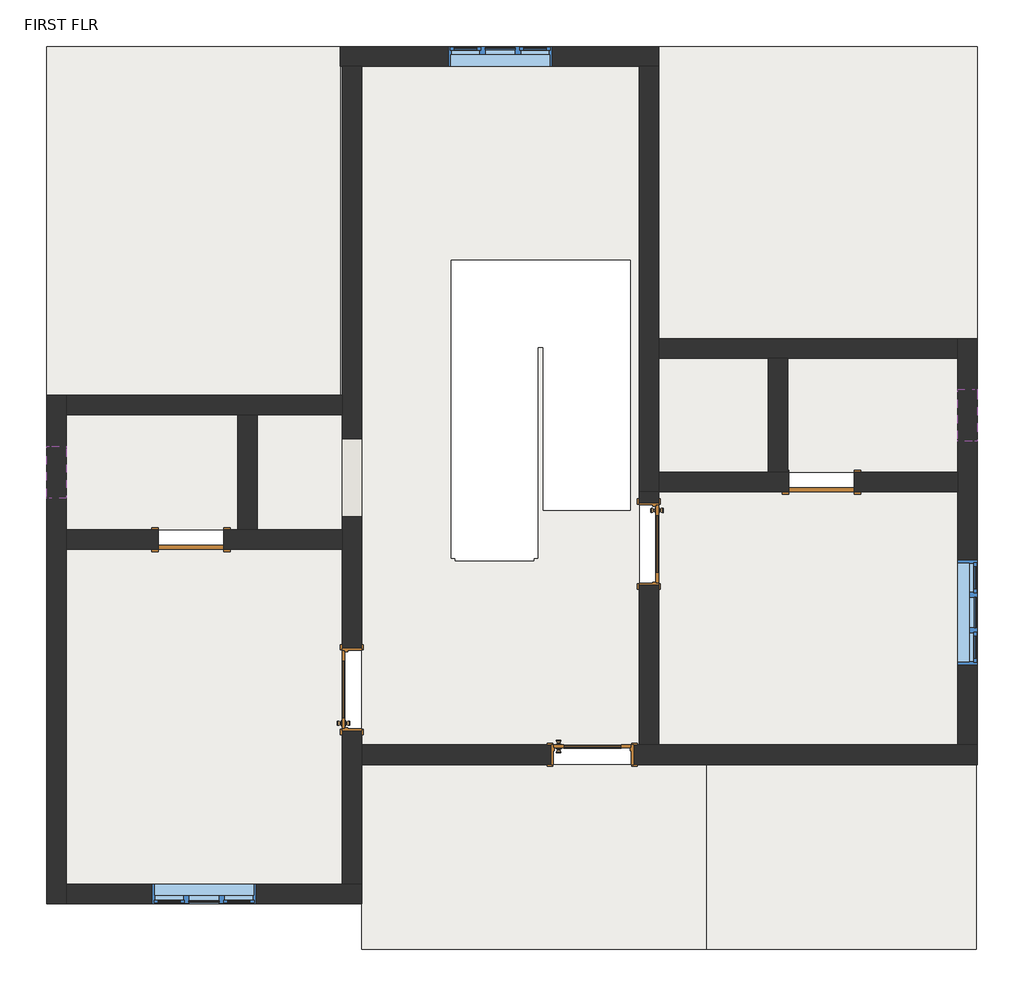
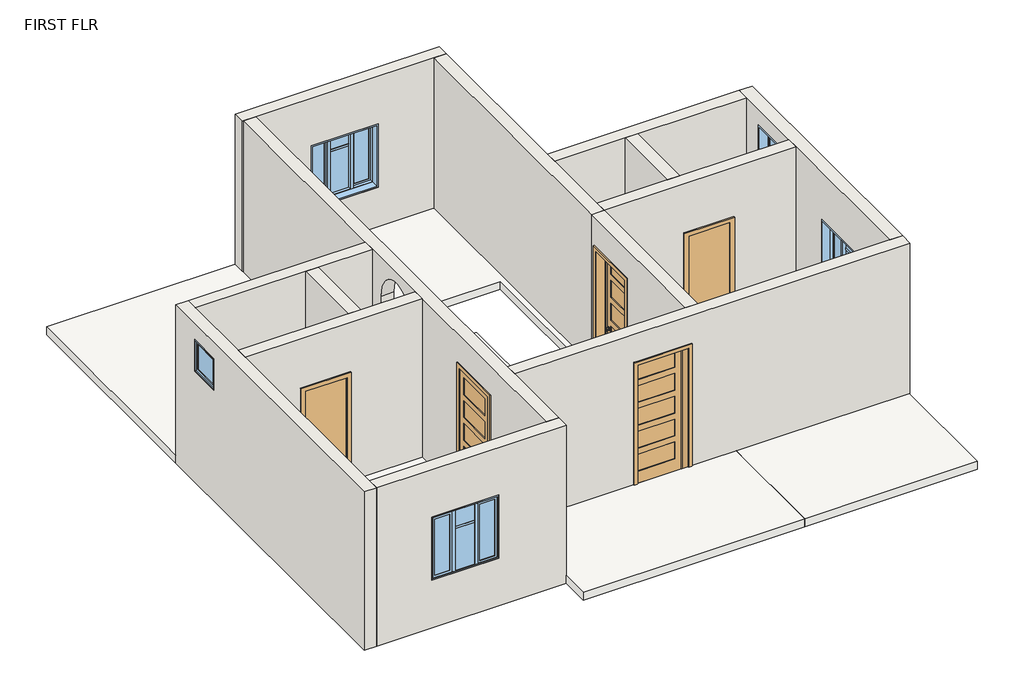
# One storey, incomplete: 14 walls, 8 slabs, 5 doors, 5 windows.
"""IFC4 building model written with IfcOpenShell, lengths in millimetres."""

from ifc_helpers import new_model, si_unit, point, frame, origin, place, context, project, spatial, polyline, ellipse_curve, trimmed, outline, extrude, faceted_brep, transform, mapped, element, save
from ifc_brep_helpers import plane_surface, extruded_surface, advanced_brep
from components import door_d793c26e, door_a1484949, window_80340324, window_casement_triple_middle_transom_window_4_x_4_1416bf83

model = new_model("IFC4")

# Units and contexts
model_context = context("Model", 3, world=origin())
ifc_project = project(units=[si_unit("LENGTHUNIT", "METRE", prefix="MILLI")], contexts=[model_context])

# Site, building, storey
site = spatial("IfcSite", under=ifc_project)
building = spatial("IfcBuilding", under=site)
storey = spatial("IfcBuildingStorey", under=building, Name="FIRST FLR", Elevation=3657.6)

# Doors
placement = place(None, origin())
door_shape = door_d793c26e(model_context)
element("IfcDoor", 1, ObjectType="Door-Interior-Single-5_Panel_Vert-Wood : 36\" x 96\"", at=placement, inside=storey, context=model_context, shape_type="MappedRepresentation", body=[
    mapped(door_shape, transform((-5771.8431792, -6106.9198807, 3657.6), x_axis=(1.0, 0.0, 0.0), y_axis=(0.0, 1.0, 0.0), z_axis=(0.0, 0.0, 1.0))),
])
element("IfcDoor", 2, ObjectType="Door-Interior-Single-5_Panel_Vert-Wood : 36\" x 96\"", at=placement, inside=storey, context=model_context, shape_type="MappedRepresentation", body=[
    mapped(door_shape, transform((-8587.0956632, -5348.0948807, 3657.6), x_axis=(0.0, 1.0, 0.0), y_axis=(-1.0, 0.0, 0.0), z_axis=(0.0, 0.0, 1.0))),
])
element("IfcDoor", 3, ObjectType="Door-Interior-Single-5_Panel_Vert-Wood : 36\" x 96\"", at=placement, inside=storey, context=model_context, shape_type="MappedRepresentation", body=[
    mapped(door_shape, transform((-5108.2681792, -3646.2948807, 3657.6), x_axis=(0.0, -1.0, 0.0), y_axis=(1.0, 0.0, 0.0), z_axis=(0.0, 0.0, 1.0))),
])
door_2_shape = door_a1484949(model_context)
element("IfcDoor", 4, ObjectType="Single-Flush : 30\" x 80\"", at=placement, inside=storey, context=model_context, shape_type="MappedRepresentation", body=[
    mapped(door_2_shape, transform((-10463.5206632, -3595.4948807, 3657.6), x_axis=(-1.0, 0.0, 0.0), y_axis=(0.0, -1.0, 0.0), z_axis=(0.0, 0.0, 1.0))),
])
element("IfcDoor", 5, ObjectType="Single-Flush : 30\" x 80\"", at=placement, inside=storey, context=model_context, shape_type="MappedRepresentation", body=[
    mapped(door_2_shape, transform((-3092.1431792, -2922.3948807, 3657.6), x_axis=(-1.0, 0.0, 0.0), y_axis=(0.0, -1.0, 0.0), z_axis=(0.0, 0.0, 1.0))),
])

# Slabs
element("IfcSlab", 6, ObjectType="GENERIC 6\"", at=placement, inside=storey, context=model_context, shape_type="SweptSolid", body=[
    extrude(outline(polyline([(-8698.2206632, -3709.7948807), (-8698.2206632, -7621.3948807), (-11924.0206632, -7621.3948807), (-11924.0206632, -3709.7948807), (-8698.2206632, -3709.7948807)])), frame((0.0, 0.0, 3505.2), z_axis=(0.0, 0.0, 1.0), x_axis=(1.0, 0.0, 0.0)), (0.0, 0.0, 1.0), 152.4),
])
element("IfcSlab", 7, ObjectType="GENERIC 6\"", at=placement, inside=storey, context=model_context, shape_type="SweptSolid", body=[
    extrude(outline(polyline([(-9917.4206632, -2134.9948807), (-9917.4206632, -3481.1948807), (-11924.0206632, -3481.1948807), (-11924.0206632, -2134.9948807), (-9917.4206632, -2134.9948807)])), frame((0.0, 0.0, 3505.2), z_axis=(0.0, 0.0, 1.0), x_axis=(1.0, 0.0, 0.0)), (0.0, 0.0, 1.0), 152.4),
])
element("IfcSlab", 8, ObjectType="GENERIC 6\"", at=placement, inside=storey, context=model_context, shape_type="SweptSolid", body=[
    extrude(outline(polyline([(-8698.2206632, -2134.9948807), (-8698.2206632, -3481.1948807), (-9688.8206632, -3481.1948807), (-9688.8206632, -2134.9948807), (-8698.2206632, -2134.9948807)])), frame((0.0, 0.0, 3505.2), z_axis=(0.0, 0.0, 1.0), x_axis=(1.0, 0.0, 0.0)), (0.0, 0.0, 1.0), 152.4),
])
element("IfcSlab", 9, ObjectType="GENERIC 6\"", at=placement, inside=storey, context=model_context, shape_type="SweptSolid", body=[
    extrude(outline(polyline([(-5225.7431792, 1941.7051193), (-5225.7431792, -5995.7948807), (-8469.6206632, -5995.7948807), (-8469.6206632, 1941.7051193), (-5225.7431792, 1941.7051193)]), holes=[polyline([(-5329.6481169, -329.5249317), (-7422.8431792, -329.5249317), (-7422.8431792, -3809.3249317), (-7372.0431792, -3809.3249317), (-7372.0431792, -3841.0749317), (-6457.6431792, -3841.0749317), (-6457.6431792, -3809.3249317), (-6406.8431792, -3809.3249317), (-6406.8431792, -1345.5249317), (-6345.6481169, -1345.5249317), (-6345.6481169, -3250.5249317), (-5329.6481169, -3250.5249317), (-5329.6481169, -329.5249317)])]), frame((0.0, 0.0, 3657.6), z_axis=(0.0, 0.0, 1.0), x_axis=(1.0, 0.0, 0.0)), (0.0, 0.0, 1.0), 152.4),
    extrude(outline(polyline([(-1497.3206632, -3036.6948807), (-1497.3206632, -5995.7948807), (-4997.1431792, -5995.7948807), (-4997.1431792, -3036.6948807), (-1497.3206632, -3036.6948807)])), frame((0.0, 0.0, 3657.6), z_axis=(0.0, 0.0, 1.0), x_axis=(1.0, 0.0, 0.0)), (0.0, 0.0, 1.0), 152.4),
    extrude(outline(polyline([(-4431.0206632, -6224.3948807), (-4431.0206632, -8383.3948807), (-8469.6206632, -8383.3948807), (-8469.6206632, -6224.3948807), (-4431.0206632, -6224.3948807)])), frame((0.0, 0.0, 3657.6), z_axis=(0.0, 0.0, 1.0), x_axis=(1.0, 0.0, 0.0)), (0.0, 0.0, 1.0), 152.4),
])
element("IfcSlab", 10, ObjectType="GENERIC 6\"", at=placement, inside=storey, context=model_context, shape_type="SweptSolid", body=[
    extrude(outline(polyline([(-1497.3206632, -1474.5948807), (-1497.3206632, -2808.0948807), (-3485.8431792, -2808.0948807), (-3485.8431792, -1474.5948807), (-1497.3206632, -1474.5948807)])), frame((0.0, 0.0, 3505.2), z_axis=(0.0, 0.0, 1.0), x_axis=(1.0, 0.0, 0.0)), (0.0, 0.0, 1.0), 152.4),
    extrude(outline(polyline([(-3714.4431792, -1474.5948807), (-3714.4431792, -2808.0948807), (-4997.1431792, -2808.0948807), (-4997.1431792, -1474.5948807), (-3714.4431792, -1474.5948807)])), frame((0.0, 0.0, 3505.2), z_axis=(0.0, 0.0, 1.0), x_axis=(1.0, 0.0, 0.0)), (0.0, 0.0, 1.0), 152.4),
])
element("IfcSlab", 11, ObjectType="GENERIC 6\"", at=placement, inside=storey, context=model_context, shape_type="SweptSolid", body=[
    extrude(outline(polyline([(-12152.6206632, 2170.3051193), (-8718.2431792, 2170.3051193), (-8718.2431792, -1906.3948807), (-12152.6206632, -1906.3948807), (-12152.6206632, 2170.3051193)])), frame((0.0, 0.0, 3657.6), z_axis=(0.0, 0.0, 1.0), x_axis=(1.0, 0.0, 0.0)), (0.0, 0.0, 1.0), 152.4),
])
element("IfcSlab", 12, ObjectType="GENERIC 6\"", at=placement, inside=storey, context=model_context, shape_type="SweptSolid", body=[
    extrude(outline(polyline([(-1268.7206632, 2170.3051193), (-1268.7206632, -1245.9948807), (-4997.1431792, -1245.9948807), (-4997.1431792, 2170.3051193), (-1268.7206632, 2170.3051193)])), frame((0.0, 0.0, 3657.6), z_axis=(0.0, 0.0, 1.0), x_axis=(1.0, 0.0, 0.0)), (0.0, 0.0, 1.0), 152.4),
])
element("IfcSlab", 13, ObjectType="GENERIC 6\"", at=placement, inside=storey, context=model_context, shape_type="SweptSolid", body=[
    extrude(outline(polyline([(-1281.4206632, -6224.3948807), (-1281.4206632, -8383.3948807), (-4431.0206632, -8383.3948807), (-4431.0206632, -6224.3948807), (-1281.4206632, -6224.3948807)])), frame((0.0, 0.0, 3657.6), z_axis=(0.0, 0.0, 1.0), x_axis=(1.0, 0.0, 0.0)), (0.0, 0.0, 1.0), 152.4),
])

# Walls
element("IfcWall", 14, ObjectType="WALL 9\"", at=placement, inside=storey, context=model_context, shape_type="Brep", body=[
    faceted_brep([(-11924.0206632, -7849.9948807, 3657.6), (-11924.0206632, -7621.3948807, 3657.6), (-11924.0206632, -3709.7948807, 3657.6), (-11924.0206632, -3481.1948807, 3657.6), (-11924.0206632, -2134.9948807, 3657.6), (-11924.0206632, -1906.3948807, 3657.6), (-11924.0206632, -1906.3948807, 6705.6), (-11924.0206632, -2134.9948807, 6705.6), (-11924.0206632, -3481.1948807, 6705.6), (-11924.0206632, -3709.7948807, 6705.6), (-11924.0206632, -7621.3948807, 6705.6), (-11924.0206632, -7849.9948807, 6705.6), (-11924.0206632, -2503.2948807, 6400.8), (-11924.0206632, -2503.2948807, 5791.2), (-11924.0206632, -3112.8948807, 5791.2), (-11924.0206632, -3112.8948807, 6400.8), (-12152.6206632, -7849.9948807, 3657.6), (-12152.6206632, -7849.9948807, 6705.6), (-12152.6206632, -1906.3948807, 6705.6), (-12152.6206632, -1906.3948807, 3657.6), (-12152.6206632, -2503.2948807, 6400.8), (-12152.6206632, -3112.8948807, 6400.8), (-12152.6206632, -3112.8948807, 5791.2), (-12152.6206632, -2503.2948807, 5791.2)], [[[0, 1, 2, 3, 4, 5, 6, 7, 8, 9, 10, 11], [12, 13, 14, 15]], [[16, 17, 18, 19], [20, 21, 22, 23]], [[5, 4, 3, 2, 1, 0, 16, 19]], [[11, 10, 9, 8, 7, 6, 18, 17]], [[0, 11, 17, 16]], [[6, 5, 19, 18]], [[13, 12, 20, 23]], [[14, 13, 23, 22]], [[15, 14, 22, 21]], [[12, 15, 21, 20]]]),
])
element("IfcWall", 15, ObjectType="WALL 9\"", at=placement, inside=storey, context=model_context, shape_type="Brep", body=[
    faceted_brep([(-11924.0206632, -7849.9948807, 3657.6), (-8469.6206632, -7849.9948807, 3657.6), (-8469.6206632, -7849.9948807, 6705.6), (-11924.0206632, -7849.9948807, 6705.6), (-10920.7206632, -7849.9948807, 5791.2), (-9701.5206632, -7849.9948807, 5791.2), (-9701.5206632, -7849.9948807, 4572.0), (-10920.7206632, -7849.9948807, 4572.0), (-11924.0206632, -7621.3948807, 3657.6), (-11924.0206632, -7621.3948807, 6705.6), (-8698.2206632, -7621.3948807, 6705.6), (-8469.6206632, -7621.3948807, 6705.6), (-8469.6206632, -7621.3948807, 3657.6), (-8698.2206632, -7621.3948807, 3657.6), (-10920.7206632, -7621.3948807, 5791.2), (-10920.7206632, -7621.3948807, 4572.0), (-9701.5206632, -7621.3948807, 4572.0), (-9701.5206632, -7621.3948807, 5791.2)], [[[0, 1, 2, 3], [4, 5, 6, 7]], [[8, 9, 10, 11, 12, 13], [14, 15, 16, 17]], [[1, 0, 8, 13, 12]], [[3, 2, 11, 10, 9]], [[0, 3, 9, 8]], [[2, 1, 12, 11]], [[15, 14, 4, 7]], [[16, 15, 7, 6]], [[17, 16, 6, 5]], [[14, 17, 5, 4]]]),
])
element("IfcWall", 16, ObjectType="WALL 9\"", at=placement, inside=storey, context=model_context, shape_type="Brep", body=[
    faceted_brep([(-11924.0206632, -2134.9948807, 3657.6), (-9917.4206632, -2134.9948807, 3657.6), (-9688.8206632, -2134.9948807, 3657.6), (-8698.2206632, -2134.9948807, 3657.6), (-8698.2206632, -2134.9948807, 6705.6), (-9688.8206632, -2134.9948807, 6705.6), (-9917.4206632, -2134.9948807, 6705.6), (-11924.0206632, -2134.9948807, 6705.6), (-11924.0206632, -1906.3948807, 3657.6), (-11924.0206632, -1906.3948807, 6705.6), (-8698.2206632, -1906.3948807, 6705.6), (-8698.2206632, -1906.3948807, 3657.6)], [[[0, 1, 2, 3, 4, 5, 6, 7]], [[8, 9, 10, 11]], [[3, 2, 1, 0, 8, 11]], [[7, 6, 5, 4, 10, 9]], [[0, 7, 9, 8]], [[4, 3, 11, 10]]]),
])
element("IfcWall", 17, ObjectType="WALL 9\"", at=placement, inside=storey, context=model_context, shape_type="Brep", body=[
    faceted_brep([(-11924.0206632, -3709.7948807, 3657.6), (-10844.5206632, -3709.7948807, 3657.6), (-10844.5206632, -3709.7948807, 5689.6), (-10082.5206632, -3709.7948807, 5689.6), (-10082.5206632, -3709.7948807, 3657.6), (-8698.2206632, -3709.7948807, 3657.6), (-8698.2206632, -3709.7948807, 6705.6), (-11924.0206632, -3709.7948807, 6705.6), (-10844.5206632, -3481.1948807, 5689.6), (-10844.5206632, -3481.1948807, 3657.6), (-11924.0206632, -3481.1948807, 3657.6), (-11924.0206632, -3481.1948807, 6705.6), (-9917.4206632, -3481.1948807, 6705.6), (-9688.8206632, -3481.1948807, 6705.6), (-8698.2206632, -3481.1948807, 6705.6), (-8698.2206632, -3481.1948807, 3657.6), (-9688.8206632, -3481.1948807, 3657.6), (-9917.4206632, -3481.1948807, 3657.6), (-10082.5206632, -3481.1948807, 3657.6), (-10082.5206632, -3481.1948807, 5689.6)], [[[0, 1, 2, 3, 4, 5, 6, 7]], [[8, 9, 10, 11, 12, 13, 14, 15, 16, 17, 18, 19]], [[10, 9, 1, 0]], [[18, 17, 16, 15, 5, 4]], [[7, 6, 14, 13, 12, 11]], [[0, 7, 11, 10]], [[6, 5, 15, 14]], [[2, 1, 9, 8]], [[3, 2, 8, 19]], [[4, 3, 19, 18]]]),
])
element("IfcWall", 18, ObjectType="WALL 9\"", at=placement, inside=storey, context=model_context, shape_type="SweptSolid", body=[
    extrude(outline(polyline([(-9917.4206632, -3481.1948807), (-9917.4206632, -2134.9948807), (-9688.8206632, -2134.9948807), (-9688.8206632, -3481.1948807), (-9917.4206632, -3481.1948807)])), frame((0.0, 0.0, 3657.6), z_axis=(0.0, 0.0, 1.0), x_axis=(1.0, 0.0, 0.0)), (0.0, 0.0, 1.0), 3048.0),
])
element("IfcWall", 19, ObjectType="WALL 9\"", at=placement, inside=storey, context=model_context, shape_type="AdvancedBrep", body=[
    advanced_brep(
    [(-8469.6206632, 1941.7051193, 6705.6), (-8469.6206632, -5995.7948807, 6705.6), (-8469.6206632, -6224.3948807, 6705.6), (-8469.6206632, -7621.3948807, 6705.6), (-8469.6206632, -7621.3948807, 3657.6), (-8469.6206632, -6224.3948807, 3657.6), (-8469.6206632, -5995.7948807, 3657.6), (-8469.6206632, -5830.6948807, 3657.6), (-8469.6206632, -5830.6948807, 6121.4), (-8469.6206632, -4865.4948807, 6121.4), (-8469.6206632, -4865.4948807, 3657.6), (-8469.6206632, 1941.7051193, 3657.6), (-8469.6206632, -3327.8747617, 5972.3014733), (-8469.6206632, -2413.4747617, 5972.3014733), (-8469.6206632, -2413.4747617, 3838.7014733), (-8469.6206632, -3327.8747617, 3838.7014733), (-8698.2206632, -7621.3948807, 6705.6), (-8698.2206632, -3709.7948807, 6705.6), (-8698.2206632, -3481.1948807, 6705.6), (-8698.2206632, -2134.9948807, 6705.6), (-8698.2206632, -1906.3948807, 6705.6), (-8698.2206632, 1941.7051193, 6705.6), (-8698.2206632, 1941.7051193, 3657.6), (-8698.2206632, -1906.3948807, 3657.6), (-8698.2206632, -2134.9948807, 3657.6), (-8698.2206632, -3481.1948807, 3657.6), (-8698.2206632, -3709.7948807, 3657.6), (-8698.2206632, -4865.4948807, 3657.6), (-8698.2206632, -4865.4948807, 6121.4), (-8698.2206632, -5830.6948807, 6121.4), (-8698.2206632, -5830.6948807, 3657.6), (-8698.2206632, -7621.3948807, 3657.6), (-8698.2206632, -2413.4747617, 5972.3014733), (-8698.2206632, -3327.8747617, 5972.3014733), (-8698.2206632, -3327.8747617, 3838.7014733), (-8698.2206632, -2413.4747617, 3838.7014733)],
    [
        (0, 1),
        (1, 2),
        (2, 3),
        (3, 4),
        (4, 5),
        (5, 6),
        (6, 7),
        (7, 8),
        (8, 9),
        (9, 10),
        (10, 11),
        (11, 0),
        (12, 13, ellipse_curve(frame((-8469.6206632, -2870.6747617, 5972.3014733), z_axis=(-1.0, 0.0, 0.0), x_axis=(0.0, 0.0, -1.0)), 533.4, 457.2)),
        (13, 14),
        (14, 15),
        (15, 12),
        (16, 17),
        (17, 18),
        (18, 19),
        (19, 20),
        (20, 21),
        (21, 22),
        (22, 23),
        (23, 24),
        (24, 25),
        (25, 26),
        (26, 27),
        (27, 28),
        (28, 29),
        (29, 30),
        (30, 31),
        (31, 16),
        (32, 33, ellipse_curve(frame((-8698.2206632, -2870.6747617, 5972.3014733), z_axis=(1.0, 0.0, 0.0), x_axis=(0.0, 0.0, -1.0)), 533.4, 457.2)),
        (33, 34),
        (34, 35),
        (35, 32),
        (3, 16),
        (31, 4),
        (11, 22),
        (21, 0),
        (9, 28),
        (27, 10),
        (8, 29),
        (7, 30),
        (12, 33),
        (32, 13),
        (35, 14),
        (34, 15),
    ],
    [
        plane_surface(frame((-8469.6206632, -7621.3948807, 3657.6), z_axis=(1.0, 0.0, 0.0), x_axis=(0.0, 1.0, 0.0))),
        plane_surface(frame((-8698.2206632, -7621.3948807, 3657.6), z_axis=(-1.0, 0.0, 0.0), x_axis=(0.0, -1.0, 0.0))),
        plane_surface(frame((-11924.0206632, -7621.3948807, 3657.6), z_axis=(0.0, -1.0, 0.0), x_axis=(-1.0, 0.0, 0.0))),
        plane_surface(frame((-8703.812186, 1941.7051193, 3657.6), z_axis=(0.0, 1.0, 0.0), x_axis=(1.0, 0.0, 0.0))),
        plane_surface(frame((-6945.6206632, -4865.4948807, 3657.6), z_axis=(0.0, -1.0, 0.0), x_axis=(-1.0, 0.0, 0.0))),
        plane_surface(frame((-6945.6206632, -4865.4948807, 6121.4), z_axis=(0.0, 0.0, -1.0), x_axis=(-1.0, 0.0, 0.0))),
        plane_surface(frame((-6945.6206632, -5830.6948807, 6121.4), z_axis=(0.0, 1.0, 0.0), x_axis=(-1.0, 0.0, 0.0))),
        plane_surface(frame((-8469.6206632, -7735.6948807, 3657.6), z_axis=(0.0, 0.0, -1.0), x_axis=(-1.0, 0.0, 0.0))),
        plane_surface(frame((-8469.6206632, 2056.0051193, 6705.6), z_axis=(0.0, 0.0, 1.0), x_axis=(-1.0, 0.0, 0.0))),
        extruded_surface(trimmed(ellipse_curve(frame((-8812.5206632, -2870.6747617, 5972.3014733), z_axis=(-1.0, 0.0, 0.0), x_axis=(0.0, 1.0, 0.0)), 457.2, 533.4), [point((-8812.5206632, -3327.8747617, 5972.3014733))], [point((-8812.5206632, -2413.4747617, 5972.3014733))], True, "CARTESIAN"), (228.60000000000036, 0.0, 0.0), 228.60000000000036),
        plane_surface(frame((-8469.6206632, -2413.4747617, 5972.3014733), z_axis=(0.0, -1.0, 0.0), x_axis=(-1.0, 0.0, 0.0))),
        plane_surface(frame((-8469.6206632, -2413.4747617, 3838.7014733), z_axis=(0.0, 0.0, 1.0), x_axis=(-1.0, 0.0, 0.0))),
        plane_surface(frame((-8469.6206632, -3327.8747617, 3838.7014733), z_axis=(0.0, 1.0, 0.0), x_axis=(-1.0, 0.0, 0.0))),
    ],
    [
        (0, [[1, 2, 3, 4, 5, 6, 7, 8, 9, 10, 11, 12], [13, 14, 15, 16]]),
        (1, [[17, 18, 19, 20, 21, 22, 23, 24, 25, 26, 27, 28, 29, 30, 31, 32], [33, 34, 35, 36]]),
        (2, [[-4, 37, -32, 38]]),
        (3, [[-12, 39, -22, 40]]),
        (4, [[41, -28, 42, -10]]),
        (5, [[-41, -9, 43, -29]]),
        (6, [[-43, -8, 44, -30]]),
        (7, [[-38, -31, -44, -7, -6, -5]]),
        (7, [[-39, -11, -42, -27, -26, -25, -24, -23]]),
        (8, [[-3, -2, -1, -40, -21, -20, -19, -18, -17, -37]]),
        (9, [[-13, 45, -33, 46]]),
        (10, [[-14, -46, -36, 47]]),
        (11, [[-15, -47, -35, 48]]),
        (12, [[-16, -48, -34, -45]]),
    ],
),
])
element("IfcWall", 20, ObjectType="WALL 9\"", at=placement, inside=storey, context=model_context, shape_type="Brep", body=[
    faceted_brep([(-8718.2431792, 1941.7051193, 3657.6), (-8698.2206632, 1941.7051193, 3657.6), (-8469.6206632, 1941.7051193, 3657.6), (-5225.7431792, 1941.7051193, 3657.6), (-4997.1431792, 1941.7051193, 3657.6), (-4997.1431792, 1941.7051193, 6705.6), (-5225.7431792, 1941.7051193, 6705.6), (-8469.6206632, 1941.7051193, 6705.6), (-8698.2206632, 1941.7051193, 6705.6), (-8718.2431792, 1941.7051193, 6705.6), (-6238.0819212, 1941.7051193, 5791.2), (-6238.0819212, 1941.7051193, 4572.0), (-7457.2819212, 1941.7051193, 4572.0), (-7457.2819212, 1941.7051193, 5791.2), (-8718.2431792, 2170.3051193, 3657.6), (-8718.2431792, 2170.3051193, 6705.6), (-4997.1431792, 2170.3051193, 6705.6), (-4997.1431792, 2170.3051193, 3657.6), (-6238.0819212, 2170.3051193, 5791.2), (-7457.2819212, 2170.3051193, 5791.2), (-7457.2819212, 2170.3051193, 4572.0), (-6238.0819212, 2170.3051193, 4572.0)], [[[0, 1, 2, 3, 4, 5, 6, 7, 8, 9], [10, 11, 12, 13]], [[14, 15, 16, 17], [18, 19, 20, 21]], [[4, 3, 2, 1, 0, 14, 17]], [[9, 8, 7, 6, 5, 16, 15]], [[0, 9, 15, 14]], [[5, 4, 17, 16]], [[11, 10, 18, 21]], [[12, 11, 21, 20]], [[13, 12, 20, 19]], [[10, 13, 19, 18]]]),
])
element("IfcWall", 21, ObjectType="WALL 9\"", at=placement, inside=storey, context=model_context, shape_type="Brep", body=[
    faceted_brep([(-5225.7431792, 1941.7051193, 3657.6), (-5225.7431792, -3036.6948807, 3657.6), (-5225.7431792, -3036.6948807, 6705.6), (-5225.7431792, 1941.7051193, 6705.6), (-4997.1431792, 1941.7051193, 3657.6), (-4997.1431792, 1941.7051193, 6705.6), (-4997.1431792, -1245.9948807, 6705.6), (-4997.1431792, -1474.5948807, 6705.6), (-4997.1431792, -2808.0948807, 6705.6), (-4997.1431792, -3036.6948807, 6705.6), (-4997.1431792, -3036.6948807, 3657.6), (-4997.1431792, -2808.0948807, 3657.6), (-4997.1431792, -1474.5948807, 3657.6), (-4997.1431792, -1245.9948807, 3657.6)], [[[0, 1, 2, 3]], [[4, 5, 6, 7, 8, 9, 10, 11, 12, 13]], [[1, 0, 4, 13, 12, 11, 10]], [[3, 2, 9, 8, 7, 6, 5]], [[0, 3, 5, 4]], [[2, 1, 10, 9]]]),
])
element("IfcWall", 22, ObjectType="WALL 9\"", at=placement, inside=storey, context=model_context, shape_type="Brep", body=[
    faceted_brep([(-1268.7206632, -6224.3948807, 6705.6), (-8469.6206632, -6224.3948807, 6705.6), (-8469.6206632, -6224.3948807, 3657.6), (-6254.4431792, -6224.3948807, 3657.6), (-6254.4431792, -6224.3948807, 6121.4), (-5289.2431792, -6224.3948807, 6121.4), (-5289.2431792, -6224.3948807, 3657.6), (-1268.7206632, -6224.3948807, 3657.6), (-8469.6206632, -5995.7948807, 6705.6), (-5225.7431792, -5995.7948807, 6705.6), (-4997.1431792, -5995.7948807, 6705.6), (-1497.3206632, -5995.7948807, 6705.6), (-1268.7206632, -5995.7948807, 6705.6), (-1268.7206632, -5995.7948807, 3657.6), (-1497.3206632, -5995.7948807, 3657.6), (-4997.1431792, -5995.7948807, 3657.6), (-5225.7431792, -5995.7948807, 3657.6), (-5289.2431792, -5995.7948807, 3657.6), (-5289.2431792, -5995.7948807, 6121.4), (-6254.4431792, -5995.7948807, 6121.4), (-6254.4431792, -5995.7948807, 3657.6), (-8469.6206632, -5995.7948807, 3657.6)], [[[0, 1, 2, 3, 4, 5, 6, 7]], [[8, 9, 10, 11, 12, 13, 14, 15, 16, 17, 18, 19, 20, 21]], [[2, 21, 20, 3]], [[13, 7, 6, 17, 16, 15, 14]], [[1, 0, 12, 11, 10, 9, 8]], [[2, 1, 8, 21]], [[0, 7, 13, 12]], [[5, 18, 17, 6]], [[18, 5, 4, 19]], [[19, 4, 3, 20]]]),
])
element("IfcWall", 23, ObjectType="WALL 9\"", at=placement, inside=storey, context=model_context, shape_type="Brep", body=[
    faceted_brep([(-4997.1431792, -3036.6948807, 3657.6), (-3473.1431792, -3036.6948807, 3657.6), (-3473.1431792, -3036.6948807, 5689.6), (-2711.1431792, -3036.6948807, 5689.6), (-2711.1431792, -3036.6948807, 3657.6), (-1497.3206632, -3036.6948807, 3657.6), (-1497.3206632, -3036.6948807, 6705.6), (-4997.1431792, -3036.6948807, 6705.6), (-3473.1431792, -2808.0948807, 5689.6), (-3473.1431792, -2808.0948807, 3657.6), (-3485.8431792, -2808.0948807, 3657.6), (-3714.4431792, -2808.0948807, 3657.6), (-4997.1431792, -2808.0948807, 3657.6), (-4997.1431792, -2808.0948807, 6705.6), (-3714.4431792, -2808.0948807, 6705.6), (-3485.8431792, -2808.0948807, 6705.6), (-1497.3206632, -2808.0948807, 6705.6), (-1497.3206632, -2808.0948807, 3657.6), (-2711.1431792, -2808.0948807, 3657.6), (-2711.1431792, -2808.0948807, 5689.6)], [[[0, 1, 2, 3, 4, 5, 6, 7]], [[8, 9, 10, 11, 12, 13, 14, 15, 16, 17, 18, 19]], [[18, 17, 5, 4]], [[12, 11, 10, 9, 1, 0]], [[7, 6, 16, 15, 14, 13]], [[0, 7, 13, 12]], [[6, 5, 17, 16]], [[2, 1, 9, 8]], [[3, 2, 8, 19]], [[4, 3, 19, 18]]]),
])
element("IfcWall", 24, ObjectType="WALL 9\"", at=placement, inside=storey, context=model_context, shape_type="Brep", body=[
    faceted_brep([(-1268.7206632, -5995.7948807, 3657.6), (-1268.7206632, -1245.9948807, 3657.6), (-1268.7206632, -1245.9948807, 6705.6), (-1268.7206632, -5995.7948807, 6705.6), (-1268.7206632, -5055.9948807, 5791.2), (-1268.7206632, -3836.7948807, 5791.2), (-1268.7206632, -3836.7948807, 4572.0), (-1268.7206632, -5055.9948807, 4572.0), (-1268.7206632, -2446.1448807, 6400.8), (-1268.7206632, -1836.5448807, 6400.8), (-1268.7206632, -1836.5448807, 5791.2), (-1268.7206632, -2446.1448807, 5791.2), (-1497.3206632, -5995.7948807, 3657.6), (-1497.3206632, -5995.7948807, 6705.6), (-1497.3206632, -3036.6948807, 6705.6), (-1497.3206632, -2808.0948807, 6705.6), (-1497.3206632, -1474.5948807, 6705.6), (-1497.3206632, -1245.9948807, 6705.6), (-1497.3206632, -1245.9948807, 3657.6), (-1497.3206632, -1474.5948807, 3657.6), (-1497.3206632, -2808.0948807, 3657.6), (-1497.3206632, -3036.6948807, 3657.6), (-1497.3206632, -5055.9948807, 5791.2), (-1497.3206632, -5055.9948807, 4572.0), (-1497.3206632, -3836.7948807, 4572.0), (-1497.3206632, -3836.7948807, 5791.2), (-1497.3206632, -2446.1448807, 6400.8), (-1497.3206632, -2446.1448807, 5791.2), (-1497.3206632, -1836.5448807, 5791.2), (-1497.3206632, -1836.5448807, 6400.8)], [[[0, 1, 2, 3], [4, 5, 6, 7], [8, 9, 10, 11]], [[12, 13, 14, 15, 16, 17, 18, 19, 20, 21], [22, 23, 24, 25], [26, 27, 28, 29]], [[1, 0, 12, 21, 20, 19, 18]], [[3, 2, 17, 16, 15, 14, 13]], [[0, 3, 13, 12]], [[2, 1, 18, 17]], [[23, 22, 4, 7]], [[24, 23, 7, 6]], [[25, 24, 6, 5]], [[22, 25, 5, 4]], [[27, 26, 8, 11]], [[28, 27, 11, 10]], [[29, 28, 10, 9]], [[26, 29, 9, 8]]]),
])
element("IfcWall", 25, ObjectType="WALL 9\"", at=placement, inside=storey, context=model_context, shape_type="Brep", body=[
    faceted_brep([(-1497.3206632, -1245.9948807, 3657.6), (-4997.1431792, -1245.9948807, 3657.6), (-4997.1431792, -1245.9948807, 6705.6), (-1497.3206632, -1245.9948807, 6705.6), (-1497.3206632, -1474.5948807, 3657.6), (-1497.3206632, -1474.5948807, 6705.6), (-3485.8431792, -1474.5948807, 6705.6), (-3714.4431792, -1474.5948807, 6705.6), (-4997.1431792, -1474.5948807, 6705.6), (-4997.1431792, -1474.5948807, 3657.6), (-3714.4431792, -1474.5948807, 3657.6), (-3485.8431792, -1474.5948807, 3657.6)], [[[0, 1, 2, 3]], [[4, 5, 6, 7, 8, 9, 10, 11]], [[1, 0, 4, 11, 10, 9]], [[3, 2, 8, 7, 6, 5]], [[0, 3, 5, 4]], [[2, 1, 9, 8]]]),
])
element("IfcWall", 26, ObjectType="WALL 9\"", at=placement, inside=storey, context=model_context, shape_type="SweptSolid", body=[
    extrude(outline(polyline([(-3714.4431792, -2808.0948807), (-3714.4431792, -1474.5948807), (-3485.8431792, -1474.5948807), (-3485.8431792, -2808.0948807), (-3714.4431792, -2808.0948807)])), frame((0.0, 0.0, 3657.6), z_axis=(0.0, 0.0, 1.0), x_axis=(1.0, 0.0, 0.0)), (0.0, 0.0, 1.0), 3048.0),
])
element("IfcWall", 27, ObjectType="WALL 9\"", at=placement, inside=storey, context=model_context, shape_type="SweptSolid", body=[
    extrude(outline(polyline([(-5995.7948807, 6705.6), (-3036.6948807, 6705.6), (-3036.6948807, 3657.6), (-3163.6948807, 3657.6), (-3163.6948807, 6121.4), (-4128.8948807, 6121.4), (-4128.8948807, 3657.6), (-5995.7948807, 3657.6), (-5995.7948807, 6705.6)])), frame((-5225.7431792, 0.0, 0.0), z_axis=(1.0, 0.0, 0.0), x_axis=(0.0, 1.0, 0.0)), (0.0, 0.0, 1.0), 228.6),
])

# Windows
window_shape = window_80340324(model_context)
element("IfcWindow", 28, ObjectType="Fixed : 24\" x 24\"", at=placement, inside=storey, context=model_context, shape_type="MappedRepresentation", body=[
    mapped(window_shape, transform((-12038.3206632, -2769.9948807, 4876.8), x_axis=(0.0, 1.0, 0.0), y_axis=(-1.0, 0.0, 0.0), z_axis=(0.0, 0.0, 1.0))),
])
element("IfcWindow", 29, ObjectType="Fixed : 24\" x 24\"", at=placement, inside=storey, context=model_context, shape_type="MappedRepresentation", body=[
    mapped(window_shape, transform((-1383.0206632, -2179.4448807, 4876.8), x_axis=(0.0, -1.0, 0.0), y_axis=(1.0, 0.0, 0.0), z_axis=(0.0, 0.0, 1.0))),
])
window_casement_triple_middle_transom_window_4_x_4_shape = window_casement_triple_middle_transom_window_4_x_4_1416bf83(model_context)
element("IfcWindow", 30, ObjectType="Window-Casement-Triple-Middle-Transom : WINDOW 4' X 4'", at=placement, inside=storey, context=model_context, shape_type="MappedRepresentation", body=[
    mapped(window_casement_triple_middle_transom_window_4_x_4_shape, transform((-10311.1206632, -7735.6948807, 3657.6), x_axis=(-1.0, 0.0, 0.0), y_axis=(0.0, -1.0, 0.0), z_axis=(0.0, 0.0, 1.0))),
])
element("IfcWindow", 31, ObjectType="Window-Casement-Triple-Middle-Transom : WINDOW 4' X 4'", at=placement, inside=storey, context=model_context, shape_type="MappedRepresentation", body=[
    mapped(window_casement_triple_middle_transom_window_4_x_4_shape, transform((-1383.0206632, -4446.3948807, 3657.6), x_axis=(0.0, -1.0, 0.0), y_axis=(1.0, 0.0, 0.0), z_axis=(0.0, 0.0, 1.0))),
])
element("IfcWindow", 32, ObjectType="Window-Casement-Triple-Middle-Transom : WINDOW 4' X 4'", at=placement, inside=storey, context=model_context, shape_type="MappedRepresentation", body=[
    mapped(window_casement_triple_middle_transom_window_4_x_4_shape, transform((-6847.6819212, 2056.0051193, 3657.6), x_axis=(1.0, 0.0, 0.0), y_axis=(0.0, 1.0, 0.0), z_axis=(0.0, 0.0, 1.0))),
])

save(model, "model.ifc")

# Revit data of these elements
# Type "Door-Interior-Single-5_Panel_Vert-Wood : 36\" x 96\""
#   Type Mark = "8"
#   Assembly Code = "C1020300"
#   Analytic Construction = "Wooden"
#   Top Rail = 0' - 4 11/16"
#   Thickness = 0' - 1 3/8"
#   Thermal Resistance (R) = 2.5876 (h·ft²·°F)/BTU
#   Swing Angle [instance default] = 90.00°
#   Stiles = 0' - 4 3/4"
#   Rough Width = 3' - 2"
#   Rough Height = 8' - 1"
#   Intermediate Rail = 0' - 4 1/2"
#   Height = 8' - 0"
#   Width = 3' - 0"
#   Heat Transfer Coefficient (U) = 0.3865 BTU/(h·ft²·°F)
#   Bottom Rail = 0' - 9 1/8"
#   Trim Material = Cherry
#   Panel Material = Cherry
#   Frame Material = Cherry
#   Door Handle Material = Aluminum
#   Visual Light Transmittance = 0
#   Solar Heat Gain Coefficient = 0
#   Wall Closure = (empty or 0)
#   Function = (empty or 0)
# Type "Single-Flush : 30\" x 80\""
#   Type Mark = "5"
#   Construction Type Id = "MDOOR"
#   Assembly Code = "C1020"
#   Analytic Construction = "Metal"
#   Thickness = 0' - 2"
#   Heat Transfer Coefficient (U) = 0.651978 BTU/(h·ft²·°F)
#   Height = 6' - 8"
#   Trim Projection Ext = 0' - 1"
#   Trim Projection Int = 0' - 1"
#   Trim Width = 0' - 3"
#   Width = 2' - 6"
#   Define Thermal Properties by = 1
#   Define Thermal Properties by = 1
#   Door Material = Door - Panel
#   Frame Material = Door - Frame
#   Visual Light Transmittance = 0
#   Solar Heat Gain Coefficient = 0
#   Function = (empty or 0)
#   Wall Closure = (empty or 0)
# Type "GENERIC 6\""
#   Assembly Code = "B1010"
#   Function = 0
#   Layers, outside or top first: 0' - 6" no material (function 1)
# Type "WALL 9\""
#   Assembly Code = "B2010"
#   Layers, outside or top first: 0' - 9" "SOFT COOL PAINT" (function 1)
# Type "Fixed : 24\" x 24\""
#   Type Mark = "3"
#   Construction Type Id = "GSP4R"
#   Assembly Code = "B2020100"
#   Analytic Construction = "1/8 in Pilkington single glazing"
#   Visual Light Transmittance = 0.9
#   Solar Heat Gain Coefficient = 0.78
#   Heat Transfer Coefficient (U) = 0.6496 BTU/(h·ft²·°F)
#   Height = 2' - 0"
#   Default Sill Height = 3' - 0"
#   Width = 2' - 0"
#   Window Inset = 0' - 0 3/4"
#   Define Thermal Properties by = 1
#   Define Thermal Properties by = 1
#   Glass Pane Material = Glass
#   Sash Material = Sash
#   Wall Closure = (empty or 0)
# Type "Window-Casement-Triple-Middle-Transom : WINDOW 4' X 4'"
#   Type Mark = "21"
#   Fire Rating = "0.5h"
#   Assembly Code = "B2020100"
#   Analytic Construction = "Double glazing - domestic"
#   Window Width = 1' - 4"
#   Window Inset [instance default] = 0' - 0 5/8"
#   Wall Thickness [instance default] = 0' - 6"
#   Visual Light Transmittance = 0.81
#   Transom Height Ratio = 0.3
#   Thermal Resistance (R) = 1.8146 (h·ft²·°F)/BTU
#   Solar Heat Gain Coefficient = 0.76
#   Rough Width = 4' - 0 1/2"
#   Rough Height = 4' - 0 1/2"
#   Heat Transfer Coefficient (U) = 0.5511 BTU/(h·ft²·°F)
#   Height = 4' - 0"
#   Transom Height = 1' - 2.4"
#   Frame Gap 3 [instance default] = 0' - 1 83/128"
#   Frame Gap 2 [instance default] = 0' - 0 5/8"
#   Frame Gap 1 = 0' - 1 51/128"
#   Default Sill Height = 3' - 0"
#   Width = 4' - 0"
#   Frame Material = WOOD MATERIAL
#   Glass Panel Material = GLASS MATERIAL
#   Wall Closure = (empty or 0)
# Elements 1, 2, 3 (IfcDoor, "Door-Interior-Single-5_Panel_Vert-Wood : 36\" x 96\"")
#   Swing Angle = 90.00°
#   Phase Created = New Construction
#   Materials on its faces: "Cherry", "Aluminum"
# Elements 4, 5 (IfcDoor, "Single-Flush : 30\" x 80\"")
#   Phase Created = New Construction
#   Materials on its faces: "Door - Frame", "Door - Panel"
# Elements 6, 7, 8, 10 (IfcSlab, "GENERIC 6\"")
#   Height Offset From Level = 0' - 0"
#   Phase Created = New Construction
#   Materials on its faces: "Default Floor"
# Elements 9, 12, 13 (IfcSlab, "GENERIC 6\"")
#   Height Offset From Level = 0' - 6"
#   Phase Created = New Construction
#   Materials on its faces: "Default Floor"
# Element 11 (IfcSlab, "GENERIC 6\"")
#   built-in parameter 1001955 = 3.14159 (stored number, unit not read)
#   Height Offset From Level = 0' - 6"
#   Phase Created = New Construction
#   Materials on its faces: "Default Floor"
# Elements 14, 15, 16, 17, 18, 19, 20, 21, 22, 23, 24, 25, 26, 27 (IfcWall, "WALL 9\"")
#   Top Offset = 0' - 0"
#   Base Offset = 0' - 0"
#   wall height = 10' - 0"
#   Phase Created = New Construction
#   Base Constraint = FIRST FLR
#   Top Constraint = Level 4
#   Materials on its faces: "SOFT COOL PAINT"
# Element 28 (IfcWindow, "Fixed : 24\" x 24\"")
#   Mark = "15"
#   Phase Created = New Construction
#   Materials on its faces: "Sash", "Glass"
# Element 29 (IfcWindow, "Fixed : 24\" x 24\"")
#   Mark = "16"
#   Phase Created = New Construction
#   Materials on its faces: "Sash", "Glass"
# Element 30 (IfcWindow, "Window-Casement-Triple-Middle-Transom : WINDOW 4' X 4'")
#   Mark = "12"
#   Window Inset = 0' - 0 5/8"
#   Frame Gap 3 = 0' - 1 83/128"
#   Frame Gap 2 = 0' - 0 5/8"
#   Phase Created = New Construction
#   Materials on its faces: "WOOD MATERIAL", "GLASS MATERIAL"
# Element 31 (IfcWindow, "Window-Casement-Triple-Middle-Transom : WINDOW 4' X 4'")
#   Mark = "13"
#   Window Inset = 0' - 0 5/8"
#   Frame Gap 3 = 0' - 1 83/128"
#   Frame Gap 2 = 0' - 0 5/8"
#   Phase Created = New Construction
#   Materials on its faces: "WOOD MATERIAL", "GLASS MATERIAL"
# Element 32 (IfcWindow, "Window-Casement-Triple-Middle-Transom : WINDOW 4' X 4'")
#   Mark = "14"
#   Window Inset = 0' - 0 5/8"
#   Frame Gap 3 = 0' - 1 83/128"
#   Frame Gap 2 = 0' - 0 5/8"
#   Phase Created = New Construction
#   Materials on its faces: "WOOD MATERIAL", "GLASS MATERIAL"
# Materials
#   "Cherry": class "Wood", colour RGB 226 177 128, transparency 0, Description = "Prunus Serotina", Cost = 0
#   "Aluminum": class "Metal", colour RGB 247 247 247, transparency 0, Description = "Aluminum 6061", Cost = 0
#   "Door - Panel": class "Wood", colour RGB 210 159 95, transparency 0, Cost = 0
#   "Door - Frame": colour RGB 118 70 51, transparency 0, Cost = 0
#   "SOFT COOL PAINT": class "Generic", colour RGB 120 120 120, transparency 0, Cost = 0
#   "Glass": class "Glass", colour RGB 0 128 192, transparency 0.75, Description = "Soda Lime Glass", Cost = 0
#   "Sash": class "Wood", colour RGB 224 178 126, transparency 0, Cost = 0
#   "WOOD MATERIAL": class "Generic", colour RGB 120 120 120, transparency 0, Cost = 0
#   "GLASS MATERIAL": class "Generic", colour RGB 120 120 120, transparency 0, Cost = 0
#   "Default Floor": colour RGB 128 128 128, transparency 0, Cost = 0
